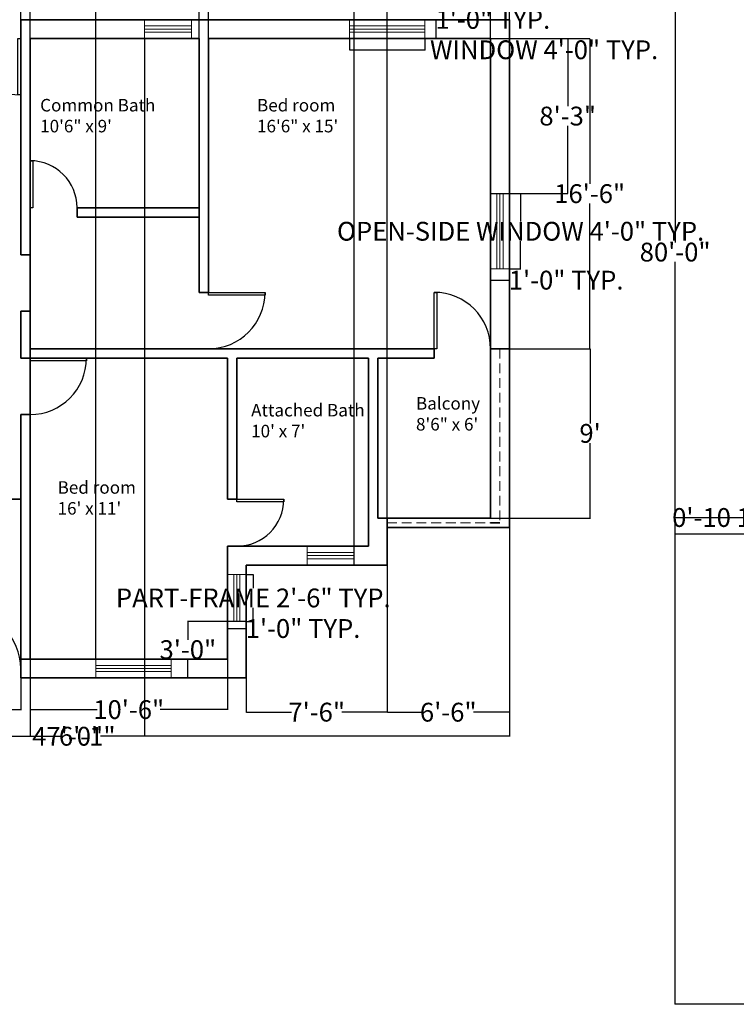
# Model space of a CAD drawing. Units: inches. Extents: x 2450 to 4494, y 1482 to 2597.
# Tile 2 of 7: x 2780 to 3238, y 1559 to 2188. Entities that reach past the tile are written whole.
import ezdxf

# ---------------------------------------------------------------- set-up
doc = ezdxf.new("R2010")
doc.units = ezdxf.units.IN
doc.header["$LTSCALE"] = 5
doc.header["$MEASUREMENT"] = 0
doc.linetypes.add('HIDDEN', pattern=[0.375, 0.25, -0.125])
for name, color, linetype, lineweight in [('A-ANNO-DIMS', 2, 'Continuous', 18), ('A-AREA-IDEN', 7, 'Continuous', 18), ('A-DOOR', 4, 'Continuous', 25), ('A-GLAZ', 4, 'Continuous', 18), ('A-WALL', 7, 'Continuous', 35), ('A-WALL-HIDN', 7, 'HIDDEN', 18)]:
    doc.layers.add(name, color=color, linetype=linetype, lineweight=lineweight)
doc.styles.get("Standard").update_dxf_attribs({"font": 'arial.ttf'})
doc.dimstyles.get("Standard").update_dxf_attribs({"dimtxt": 12, "dimasz": 0.18, "dimexe": 0.18, "dimexo": 0.0625, "dimgap": 0.09, "dimtad": 0, "dimtih": 1, "dimtoh": 1, "dimdec": 0, "dimzin": 0, "dimdsep": 46, "dimlunit": 3, "dimtxsty": 'Standard', "dimcen": 0.09, "dimadec": 0, "dimazin": 0, "dimtfac": 1, "dimtdec": 0, "dimtofl": 0, "dimtmove": 0, "dimatfit": 3, "dimfxl": 1, "dimtolj": 1, "dimtzin": 0, "dimarcsym": 0})

# ---------------------------------------------------------------- blocks, each defined once
blk = doc.blocks.new('*U2')
for p, q in [((0, 0), (0, -6)), ((36, 0), (36, -6))]:
    blk.add_line(p, q)
blk.add_lwpolyline([(0, 0), (0, 36), (1.75, 36), (1.75, 0)], close=True)
blk.add_arc((0, 0), 36, 0, 90)
blk = doc.blocks.new('*U3')
for p, q in [((0, 0), (0, -6)), ((30, 0), (30, -6))]:
    blk.add_line(p, q)
blk.add_lwpolyline([(0, 0), (0, 30), (1.75, 30), (1.75, 0)], close=True)
blk.add_arc((0, 0), 30, 0, 90)
blk = doc.blocks.new('*U5')
for p, q in [((-36, 0), (-36, 6)), ((0, 0), (0, 6))]:
    blk.add_line(p, q)
blk.add_lwpolyline([(0, 0), (0, -36), (-1.75, -36), (-1.75, 0)], close=True)
blk.add_arc((0, 0), 36, 180, 270)
blk = doc.blocks.new('*D6')
at = {"layer": 'A-ANNO-DIMS', "color": 0, "lineweight": -2, "ltscale": 5, "transparency": 16777216}
for p, q in [((2900.93, 2175.63), (2900.93, 2236.59)), ((2901.11, 2236.41), (2981.22, 2236.41)), ((3080.75, 2236.41), (3000.64, 2236.41)), ((3080.93, 2175.63), (3080.93, 2236.59))]:
    blk.add_line(p, q, dxfattribs=at)
at = {"layer": 'A-ANNO-DIMS', "color": 0, "ltscale": 5, "transparency": 16777216}
for points in [[(2901.11, 2236.44), (2901.11, 2236.38), (2900.93, 2236.41)], [(3080.75, 2236.44), (3080.75, 2236.38), (3080.93, 2236.41)]]:
    blk.add_solid(points, dxfattribs=at)
at = {"layer": 'Defpoints', "color": 0, "ltscale": 5, "transparency": 16777216}
for p in [(3080.93, 2236.41), (2900.93, 2175.57), (3080.93, 2175.57)]:
    blk.add_point(p, dxfattribs=at)
at = {"layer": 'A-ANNO-DIMS', "color": 0, "ltscale": 5, "transparency": 16777216, "insert": (2990.93, 2236.41), "char_height": 12, "attachment_point": 5}
blk.add_mtext("\\A1;15'", dxfattribs=at)
blk = doc.blocks.new('*D7')
at = {"layer": 'A-ANNO-DIMS', "color": 0, "lineweight": -2, "ltscale": 5, "transparency": 16777216}
for p, q in [((3080.93, 2175.63), (3080.93, 2236.59)), ((3081.11, 2236.41), (3081.88, 2236.41)), ((3092.75, 2236.41), (3091.98, 2236.41)), ((3092.93, 2175.63), (3092.93, 2236.59))]:
    blk.add_line(p, q, dxfattribs=at)
at = {"layer": 'A-ANNO-DIMS', "color": 0, "ltscale": 5, "transparency": 16777216}
for points in [[(3081.11, 2236.44), (3081.11, 2236.38), (3080.93, 2236.41)], [(3092.75, 2236.44), (3092.75, 2236.38), (3092.93, 2236.41)]]:
    blk.add_solid(points, dxfattribs=at)
at = {"layer": 'Defpoints', "color": 0, "ltscale": 5, "transparency": 16777216}
for p in [(3092.93, 2236.41), (3080.93, 2175.57), (3092.93, 2175.57)]:
    blk.add_point(p, dxfattribs=at)
at = {"layer": 'A-ANNO-DIMS', "color": 0, "ltscale": 5, "transparency": 16777216, "insert": (3086.93, 2236.41), "char_height": 12, "attachment_point": 5}
blk.add_mtext("\\A1;1'", dxfattribs=at)
blk = doc.blocks.new('*D8')
at = {"layer": 'A-ANNO-DIMS', "color": 0, "lineweight": -2, "ltscale": 5, "transparency": 16777216}
for p, q in [((2786.93, 2175.63), (2786.93, 2236.19)), ((2787.11, 2236.01), (2835.32, 2236.01)), ((2894.75, 2236.01), (2846.54, 2236.01)), ((2894.93, 2175.63), (2894.93, 2236.19))]:
    blk.add_line(p, q, dxfattribs=at)
at = {"layer": 'A-ANNO-DIMS', "color": 0, "ltscale": 5, "transparency": 16777216}
for points in [[(2787.11, 2236.04), (2787.11, 2235.98), (2786.93, 2236.01)], [(2894.75, 2236.04), (2894.75, 2235.98), (2894.93, 2236.01)]]:
    blk.add_solid(points, dxfattribs=at)
at = {"layer": 'Defpoints', "color": 0, "ltscale": 5, "transparency": 16777216}
for p in [(2894.93, 2236.01), (2786.93, 2175.57), (2894.93, 2175.57)]:
    blk.add_point(p, dxfattribs=at)
at = {"layer": 'A-ANNO-DIMS', "color": 0, "ltscale": 5, "transparency": 16777216, "insert": (2840.93, 2236.01), "char_height": 12, "attachment_point": 5}
blk.add_mtext("\\A1;9'", dxfattribs=at)
blk = doc.blocks.new('*D9')
at = {"layer": 'A-ANNO-DIMS', "color": 0, "lineweight": -2, "ltscale": 5, "transparency": 16777216}
for p, q in [((2894.93, 2175.63), (2894.93, 2251.28)), ((2895.11, 2251.1), (2900.75, 2251.1)), ((2900.93, 2175.63), (2900.93, 2251.28)), ((2900.93, 2251.1), (2901.11, 2251.1))]:
    blk.add_line(p, q, dxfattribs=at)
at = {"layer": 'A-ANNO-DIMS', "color": 0, "ltscale": 5, "transparency": 16777216}
for points in [[(2895.11, 2251.13), (2895.11, 2251.07), (2894.93, 2251.1)], [(2900.75, 2251.13), (2900.75, 2251.07), (2900.93, 2251.1)]]:
    blk.add_solid(points, dxfattribs=at)
at = {"layer": 'Defpoints', "color": 0, "ltscale": 5, "transparency": 16777216}
for p in [(2900.93, 2251.1), (2894.93, 2175.57), (2900.93, 2175.57)]:
    blk.add_point(p, dxfattribs=at)
at = {"layer": 'A-ANNO-DIMS', "color": 0, "ltscale": 5, "transparency": 16777216, "insert": (2908.13, 2251.1), "char_height": 12, "attachment_point": 5}
blk.add_mtext('\\A1;6"', dxfattribs=at)
blk = doc.blocks.new('*D10')
at = {"layer": 'A-ANNO-DIMS', "color": 0, "lineweight": -2, "ltscale": 5, "transparency": 16777216}
for p, q in [((2648.93, 2175.63), (2648.93, 2236.37)), ((2649.11, 2236.19), (2705.22, 2236.19)), ((2780.75, 2236.19), (2724.64, 2236.19)), ((2780.93, 2175.63), (2780.93, 2236.37))]:
    blk.add_line(p, q, dxfattribs=at)
at = {"layer": 'A-ANNO-DIMS', "color": 0, "ltscale": 5, "transparency": 16777216}
for points in [[(2649.11, 2236.22), (2649.11, 2236.16), (2648.93, 2236.19)], [(2780.75, 2236.22), (2780.75, 2236.16), (2780.93, 2236.19)]]:
    blk.add_solid(points, dxfattribs=at)
at = {"layer": 'Defpoints', "color": 0, "ltscale": 5, "transparency": 16777216}
for p in [(2780.93, 2236.19), (2648.93, 2175.57), (2780.93, 2175.57)]:
    blk.add_point(p, dxfattribs=at)
at = {"layer": 'A-ANNO-DIMS', "color": 0, "ltscale": 5, "transparency": 16777216, "insert": (2714.93, 2236.19), "char_height": 12, "attachment_point": 5}
blk.add_mtext("\\A1;11'", dxfattribs=at)
blk = doc.blocks.new('*D18')
at = {"layer": 'A-ANNO-DIMS', "color": 0, "lineweight": -2, "ltscale": 5, "transparency": 16777216}
for p, q in [((2648.93, 1779.51), (2648.93, 1747)), ((2780.93, 1779.51), (2780.93, 1747)), ((2649.11, 1747.18), (2705.22, 1747.18)), ((2780.75, 1747.18), (2724.64, 1747.18))]:
    blk.add_line(p, q, dxfattribs=at)
at = {"layer": 'A-ANNO-DIMS', "color": 0, "ltscale": 5, "transparency": 16777216}
for points in [[(2649.11, 1747.21), (2649.11, 1747.15), (2648.93, 1747.18)], [(2780.75, 1747.21), (2780.75, 1747.15), (2780.93, 1747.18)]]:
    blk.add_solid(points, dxfattribs=at)
at = {"layer": 'Defpoints', "color": 0, "ltscale": 5, "transparency": 16777216}
for p in [(2648.93, 1779.57), (2780.93, 1779.57), (2648.93, 1747.18)]:
    blk.add_point(p, dxfattribs=at)
at = {"layer": 'A-ANNO-DIMS', "color": 0, "ltscale": 5, "transparency": 16777216, "insert": (2714.93, 1747.18), "char_height": 12, "attachment_point": 5}
blk.add_mtext("\\A1;11'", dxfattribs=at)
blk = doc.blocks.new('*D19')
at = {"layer": 'A-ANNO-DIMS', "color": 0, "lineweight": -2, "ltscale": 5, "transparency": 16777216}
for p, q in [((2786.93, 1779.51), (2786.93, 1747.15)), ((2912.93, 1779.51), (2912.93, 1747.15)), ((2787.11, 1747.33), (2829.79, 1747.33)), ((2912.75, 1747.33), (2870.07, 1747.33))]:
    blk.add_line(p, q, dxfattribs=at)
at = {"layer": 'A-ANNO-DIMS', "color": 0, "ltscale": 5, "transparency": 16777216}
for points in [[(2787.11, 1747.36), (2787.11, 1747.3), (2786.93, 1747.33)], [(2912.75, 1747.36), (2912.75, 1747.3), (2912.93, 1747.33)]]:
    blk.add_solid(points, dxfattribs=at)
at = {"layer": 'Defpoints', "color": 0, "ltscale": 5, "transparency": 16777216}
for p in [(2786.93, 1779.57), (2912.93, 1779.57), (2912.93, 1747.33)]:
    blk.add_point(p, dxfattribs=at)
at = {"layer": 'A-ANNO-DIMS', "color": 0, "ltscale": 5, "transparency": 16777216, "insert": (2849.93, 1747.33), "char_height": 12, "attachment_point": 5}
blk.add_mtext('\\A1;10\'-6"', dxfattribs=at)
blk = doc.blocks.new('*D20')
at = {"layer": 'A-ANNO-DIMS', "color": 0, "lineweight": -2, "ltscale": 5, "transparency": 16777216}
for p, q in [((2924.93, 1839.51), (2924.93, 1745.52)), ((3014.93, 1839.51), (3014.93, 1745.52)), ((2925.11, 1745.7), (2953.94, 1745.7)), ((3014.75, 1745.7), (2985.92, 1745.7))]:
    blk.add_line(p, q, dxfattribs=at)
at = {"layer": 'A-ANNO-DIMS', "color": 0, "ltscale": 5, "transparency": 16777216}
for points in [[(2925.11, 1745.73), (2925.11, 1745.67), (2924.93, 1745.7)], [(3014.75, 1745.73), (3014.75, 1745.67), (3014.93, 1745.7)]]:
    blk.add_solid(points, dxfattribs=at)
at = {"layer": 'Defpoints', "color": 0, "ltscale": 5, "transparency": 16777216}
for p in [(2924.93, 1839.57), (3014.93, 1839.57), (3014.93, 1745.7)]:
    blk.add_point(p, dxfattribs=at)
at = {"layer": 'A-ANNO-DIMS', "color": 0, "ltscale": 5, "transparency": 16777216, "insert": (2969.93, 1745.7), "char_height": 12, "attachment_point": 5}
blk.add_mtext('\\A1;7\'-6"', dxfattribs=at)
blk = doc.blocks.new('*D21')
at = {"layer": 'A-ANNO-DIMS', "color": 0, "lineweight": -2, "ltscale": 5, "transparency": 16777216}
for p, q in [((3014.93, 1863.51), (3014.93, 1745.49)), ((3092.93, 1863.51), (3092.93, 1745.49)), ((3015.11, 1745.67), (3037.86, 1745.67)), ((3092.75, 1745.67), (3070, 1745.67))]:
    blk.add_line(p, q, dxfattribs=at)
at = {"layer": 'A-ANNO-DIMS', "color": 0, "ltscale": 5, "transparency": 16777216}
for points in [[(3015.11, 1745.7), (3015.11, 1745.64), (3014.93, 1745.67)], [(3092.75, 1745.7), (3092.75, 1745.64), (3092.93, 1745.67)]]:
    blk.add_solid(points, dxfattribs=at)
at = {"layer": 'Defpoints', "color": 0, "ltscale": 5, "transparency": 16777216}
for p in [(3014.93, 1863.57), (3092.93, 1863.57), (3014.93, 1745.67)]:
    blk.add_point(p, dxfattribs=at)
at = {"layer": 'A-ANNO-DIMS', "color": 0, "ltscale": 5, "transparency": 16777216, "insert": (3053.93, 1745.67), "char_height": 12, "attachment_point": 5}
blk.add_mtext('\\A1;6\'-6"', dxfattribs=at)
blk = doc.blocks.new('*D22')
at = {"layer": 'A-ANNO-DIMS', "color": 0, "lineweight": -2, "ltscale": 5, "transparency": 16777216}
for p, q in [((3080.99, 1977.57), (3144.66, 1977.57)), ((3144.48, 1977.39), (3144.48, 1929.79)), ((3144.48, 1869.75), (3144.48, 1917.35)), ((3080.99, 1869.57), (3144.66, 1869.57))]:
    blk.add_line(p, q, dxfattribs=at)
at = {"layer": 'A-ANNO-DIMS', "color": 0, "ltscale": 5, "transparency": 16777216}
for points in [[(3144.45, 1977.39), (3144.51, 1977.39), (3144.48, 1977.57)], [(3144.45, 1869.75), (3144.51, 1869.75), (3144.48, 1869.57)]]:
    blk.add_solid(points, dxfattribs=at)
at = {"layer": 'Defpoints', "color": 0, "ltscale": 5, "transparency": 16777216}
for p in [(3080.93, 1977.57), (3144.48, 1977.57), (3080.93, 1869.57)]:
    blk.add_point(p, dxfattribs=at)
at = {"layer": 'A-ANNO-DIMS', "color": 0, "ltscale": 5, "transparency": 16777216, "insert": (3144.48, 1923.57), "char_height": 12, "attachment_point": 5}
blk.add_mtext("\\A1;9'", dxfattribs=at)
blk = doc.blocks.new('*D23')
at = {"layer": 'A-ANNO-DIMS', "color": 0, "lineweight": -2, "ltscale": 5, "transparency": 16777216}
for p, q in [((3080.99, 2175.57), (3144.41, 2175.57)), ((3144.23, 2175.39), (3144.23, 2082.79)), ((3144.23, 1977.75), (3144.23, 2070.35)), ((3080.99, 1977.57), (3144.41, 1977.57))]:
    blk.add_line(p, q, dxfattribs=at)
at = {"layer": 'A-ANNO-DIMS', "color": 0, "ltscale": 5, "transparency": 16777216}
for points in [[(3144.2, 2175.39), (3144.26, 2175.39), (3144.23, 2175.57)], [(3144.2, 1977.75), (3144.26, 1977.75), (3144.23, 1977.57)]]:
    blk.add_solid(points, dxfattribs=at)
at = {"layer": 'Defpoints', "color": 0, "ltscale": 5, "transparency": 16777216}
for p in [(3080.93, 2175.57), (3080.93, 1977.57), (3144.23, 1977.57)]:
    blk.add_point(p, dxfattribs=at)
at = {"layer": 'A-ANNO-DIMS', "color": 0, "ltscale": 5, "transparency": 16777216, "insert": (3144.23, 2076.57), "char_height": 12, "attachment_point": 5}
blk.add_mtext('\\A1;16\'-6"', dxfattribs=at)
blk = doc.blocks.new('WIN-30-FRAME')
for p, q in [((0, 0), (0, 12)), ((0, 12), (30, 12)), ((30, 8), (0, 8)), ((30, 12), (30, 0)), ((30, 6), (0, 6)), ((30, 4), (0, 4)), ((30, 0), (0, 0))]:
    blk.add_line(p, q)
blk = doc.blocks.new('WIN-48-FRAME')
for p, q in [((48, 12), (0, 12)), ((0, 12), (0, 0)), ((48, 8), (0, 8)), ((48, 0), (48, 12)), ((48, 6), (0, 6)), ((48, 4), (0, 4)), ((0, 0), (48, 0))]:
    blk.add_line(p, q)
blk = doc.blocks.new('WIN-30-PART-FRAME')
for p, q in [((12, 30), (0, 30)), ((0, 30), (0, 0)), ((4, 30), (4, 0)), ((6, 30), (6, 0)), ((8, 30), (8, 0)), ((12, 6), (12, 30)), ((0, 0), (12, 0))]:
    blk.add_line(p, q)
blk = doc.blocks.new('WIN-48-PART-FRAME')
for p, q in [((48, 12), (0, 12)), ((0, 12), (0, 0)), ((48, 8), (0, 8)), ((48, 0), (48, 12)), ((48, 6), (0, 6)), ((48, 4), (0, 4)), ((24, 0), (48, 0))]:
    blk.add_line(p, q)
blk = doc.blocks.new('WIN-48-OPEN-SIDE')
for p, q in [((0, 48), (12, 48)), ((4, 48), (4, 0)), ((6, 48), (6, 0)), ((8, 48), (8, 0)), ((12, 48), (12, 0)), ((12, 0), (0, 0))]:
    blk.add_line(p, q)
blk = doc.blocks.new('*D41')
at = {"layer": 'A-ANNO-DIMS', "color": 0, "lineweight": -2, "ltscale": 5, "transparency": 16777216}
for p, q in [((2990.93, 2175.51), (2990.93, 2168.19)), ((3038.93, 2175.51), (3038.93, 2168.19)), ((2991.11, 2168.37), (3038.75, 2168.37)), ((3038.93, 2168.37), (3039.11, 2168.37))]:
    blk.add_line(p, q, dxfattribs=at)
at = {"layer": 'A-ANNO-DIMS', "color": 0, "ltscale": 5, "transparency": 16777216}
for points in [[(2991.11, 2168.4), (2991.11, 2168.34), (2990.93, 2168.37)], [(3038.75, 2168.4), (3038.75, 2168.34), (3038.93, 2168.37)]]:
    blk.add_solid(points, dxfattribs=at)
at = {"layer": 'Defpoints', "color": 0, "ltscale": 5, "transparency": 16777216}
for p in [(2990.93, 2175.57), (3038.93, 2175.57), (3038.93, 2168.37)]:
    blk.add_point(p, dxfattribs=at)
at = {"layer": 'A-ANNO-DIMS', "color": 0, "ltscale": 5, "transparency": 16777216, "insert": (3115.13, 2168.37), "char_height": 12, "attachment_point": 5}
blk.add_mtext('\\A1;WINDOW 4\'-0" TYP.', dxfattribs=at)
blk = doc.blocks.new('*D42')
at = {"layer": 'A-ANNO-DIMS', "color": 0, "lineweight": -2, "ltscale": 5, "transparency": 16777216}
for p, q in [((3038.99, 2187.57), (3046.31, 2187.57)), ((3046.13, 2187.57), (3046.13, 2187.75)), ((3046.13, 2187.75), (3046.31, 2187.75)), ((3046.13, 2175.75), (3046.13, 2187.39)), ((3038.99, 2175.57), (3046.31, 2175.57))]:
    blk.add_line(p, q, dxfattribs=at)
at = {"layer": 'A-ANNO-DIMS', "color": 0, "ltscale": 5, "transparency": 16777216}
for points in [[(3046.1, 2187.39), (3046.16, 2187.39), (3046.13, 2187.57)], [(3046.1, 2175.75), (3046.16, 2175.75), (3046.13, 2175.57)]]:
    blk.add_solid(points, dxfattribs=at)
at = {"layer": 'Defpoints', "color": 0, "ltscale": 5, "transparency": 16777216}
for p in [(3038.93, 2187.57), (3046.13, 2187.57), (3038.93, 2175.57)]:
    blk.add_point(p, dxfattribs=at)
at = {"layer": 'A-ANNO-DIMS', "color": 0, "ltscale": 5, "transparency": 16777216, "insert": (3082.41, 2187.75), "char_height": 12, "attachment_point": 5}
blk.add_mtext('\\A1;1\'-0" TYP.', dxfattribs=at)
blk = doc.blocks.new('*D43')
at = {"layer": 'A-ANNO-DIMS', "color": 0, "lineweight": -2, "ltscale": 5, "transparency": 16777216}
for p, q in [((2924.99, 1833.57), (2929.61, 1833.57)), ((2929.43, 1833.39), (2929.43, 1824.79)), ((2929.43, 1803.75), (2929.43, 1812.35)), ((2924.99, 1803.57), (2929.61, 1803.57))]:
    blk.add_line(p, q, dxfattribs=at)
at = {"layer": 'A-ANNO-DIMS', "color": 0, "ltscale": 5, "transparency": 16777216}
for points in [[(2929.4, 1833.39), (2929.46, 1833.39), (2929.43, 1833.57)], [(2929.4, 1803.75), (2929.46, 1803.75), (2929.43, 1803.57)]]:
    blk.add_solid(points, dxfattribs=at)
at = {"layer": 'Defpoints', "color": 0, "ltscale": 5, "transparency": 16777216}
for p in [(2924.93, 1833.57), (2929.43, 1833.57), (2924.93, 1803.57)]:
    blk.add_point(p, dxfattribs=at)
at = {"layer": 'A-ANNO-DIMS', "color": 0, "ltscale": 5, "transparency": 16777216, "insert": (2929.43, 1818.57), "char_height": 12, "attachment_point": 5}
blk.add_mtext('\\A1;PART-FRAME 2\'-6" TYP.', dxfattribs=at)
blk = doc.blocks.new('*D44')
at = {"layer": 'A-ANNO-DIMS', "color": 0, "lineweight": -2, "ltscale": 5, "transparency": 16777216}
for p, q in [((2912.93, 1803.51), (2912.93, 1798.89)), ((2924.93, 1803.51), (2924.93, 1798.89)), ((2913.11, 1799.07), (2924.75, 1799.07)), ((2924.93, 1799.07), (2925.11, 1799.07))]:
    blk.add_line(p, q, dxfattribs=at)
at = {"layer": 'A-ANNO-DIMS', "color": 0, "ltscale": 5, "transparency": 16777216}
for points in [[(2913.11, 1799.1), (2913.11, 1799.04), (2912.93, 1799.07)], [(2924.75, 1799.1), (2924.75, 1799.04), (2924.93, 1799.07)]]:
    blk.add_solid(points, dxfattribs=at)
at = {"layer": 'Defpoints', "color": 0, "ltscale": 5, "transparency": 16777216}
for p in [(2912.93, 1803.57), (2924.93, 1803.57), (2924.93, 1799.07)]:
    blk.add_point(p, dxfattribs=at)
at = {"layer": 'A-ANNO-DIMS', "color": 0, "ltscale": 5, "transparency": 16777216, "insert": (2961.21, 1799.07), "char_height": 12, "attachment_point": 5}
blk.add_mtext('\\A1;1\'-0" TYP.', dxfattribs=at)
blk = doc.blocks.new('*D47')
at = {"layer": 'A-ANNO-DIMS', "color": 0, "lineweight": -2, "ltscale": 5, "transparency": 16777216}
for p, q in [((3092.99, 2076.57), (3100.31, 2076.57)), ((3100.13, 2076.39), (3100.13, 2058.87)), ((3100.13, 2028.75), (3100.13, 2046.27)), ((3092.99, 2028.57), (3100.31, 2028.57))]:
    blk.add_line(p, q, dxfattribs=at)
at = {"layer": 'A-ANNO-DIMS', "color": 0, "ltscale": 5, "transparency": 16777216}
for points in [[(3100.1, 2076.39), (3100.16, 2076.39), (3100.13, 2076.57)], [(3100.1, 2028.75), (3100.16, 2028.75), (3100.13, 2028.57)]]:
    blk.add_solid(points, dxfattribs=at)
at = {"layer": 'Defpoints', "color": 0, "ltscale": 5, "transparency": 16777216}
for p in [(3092.93, 2076.57), (3100.13, 2076.57), (3092.93, 2028.57)]:
    blk.add_point(p, dxfattribs=at)
at = {"layer": 'A-ANNO-DIMS', "color": 0, "ltscale": 5, "transparency": 16777216, "insert": (3100.13, 2052.57), "char_height": 12, "attachment_point": 5}
blk.add_mtext('\\A1;OPEN-SIDE WINDOW 4\'-0" TYP.', dxfattribs=at)
blk = doc.blocks.new('*D48')
at = {"layer": 'A-ANNO-DIMS', "color": 0, "lineweight": -2, "ltscale": 5, "transparency": 16777216}
for p, q in [((3080.93, 2028.51), (3080.93, 2021.19)), ((3092.93, 2028.51), (3092.93, 2021.19)), ((3081.11, 2021.37), (3092.75, 2021.37)), ((3092.93, 2021.37), (3093.11, 2021.37))]:
    blk.add_line(p, q, dxfattribs=at)
at = {"layer": 'A-ANNO-DIMS', "color": 0, "ltscale": 5, "transparency": 16777216}
for points in [[(3081.11, 2021.4), (3081.11, 2021.34), (3080.93, 2021.37)], [(3092.75, 2021.4), (3092.75, 2021.34), (3092.93, 2021.37)]]:
    blk.add_solid(points, dxfattribs=at)
at = {"layer": 'Defpoints', "color": 0, "ltscale": 5, "transparency": 16777216}
for p in [(3080.93, 2028.57), (3092.93, 2028.57), (3092.93, 2021.37)]:
    blk.add_point(p, dxfattribs=at)
at = {"layer": 'A-ANNO-DIMS', "color": 0, "ltscale": 5, "transparency": 16777216, "insert": (3129.21, 2021.37), "char_height": 12, "attachment_point": 5}
blk.add_mtext('\\A1;1\'-0" TYP.', dxfattribs=at)
blk = doc.blocks.new('*D69')
at = {"layer": 'A-ANNO-DIMS', "color": 0, "lineweight": -2, "ltscale": 5, "transparency": 16777216}
for p, q in [((2528.93, 1869.51), (2528.93, 1730.14)), ((3092.93, 1863.51), (3092.93, 1730.14)), ((2529.11, 1730.32), (2789.99, 1730.32)), ((3092.75, 1730.32), (2831.87, 1730.32))]:
    blk.add_line(p, q, dxfattribs=at)
at = {"layer": 'A-ANNO-DIMS', "color": 0, "ltscale": 5, "transparency": 16777216}
for points in [[(2529.11, 1730.35), (2529.11, 1730.29), (2528.93, 1730.32)], [(3092.75, 1730.35), (3092.75, 1730.29), (3092.93, 1730.32)]]:
    blk.add_solid(points, dxfattribs=at)
at = {"layer": 'Defpoints', "color": 0, "ltscale": 5, "transparency": 16777216}
for p in [(2528.93, 1869.57), (3092.93, 1863.57), (3092.93, 1730.32)]:
    blk.add_point(p, dxfattribs=at)
at = {"layer": 'A-ANNO-DIMS', "color": 0, "ltscale": 5, "transparency": 16777216, "insert": (2810.93, 1730.32), "char_height": 12, "attachment_point": 5}
blk.add_mtext('\\A1;47\'-0"', dxfattribs=at)
blk = doc.blocks.new('*D72')
at = {"layer": 'A-ANNO-DIMS', "color": 0, "lineweight": -2, "ltscale": 5, "transparency": 16777216}
for p, q in [((3426.23, 2519.27), (3198.61, 2519.27)), ((3198.79, 2519.09), (3198.79, 2045.48)), ((3198.79, 1559.45), (3198.79, 2033.05)), ((3426.23, 1559.27), (3198.61, 1559.27))]:
    blk.add_line(p, q, dxfattribs=at)
at = {"layer": 'A-ANNO-DIMS', "color": 0, "ltscale": 5, "transparency": 16777216}
for points in [[(3198.76, 2519.09), (3198.82, 2519.09), (3198.79, 2519.27)], [(3198.76, 1559.45), (3198.82, 1559.45), (3198.79, 1559.27)]]:
    blk.add_solid(points, dxfattribs=at)
at = {"layer": 'Defpoints', "color": 0, "ltscale": 5, "transparency": 16777216}
for p in [(3198.79, 2519.27), (3426.29, 2519.27), (3426.29, 1559.27)]:
    blk.add_point(p, dxfattribs=at)
at = {"layer": 'A-ANNO-DIMS', "color": 0, "ltscale": 5, "transparency": 16777216, "insert": (3198.79, 2039.27), "char_height": 12, "attachment_point": 5}
blk.add_mtext('\\A1;80\'-0"', dxfattribs=at)
blk = doc.blocks.new('*D76')
at = {"layer": 'A-ANNO-DIMS', "color": 0, "lineweight": -2, "ltscale": 5, "transparency": 16777216}
for p, q in [((2786.93, 2175.51), (2786.93, 1730.14)), ((2859.92, 2175.51), (2859.92, 1730.14)), ((2787.11, 1730.32), (2807.35, 1730.32)), ((2859.74, 1730.32), (2839.5, 1730.32))]:
    blk.add_line(p, q, dxfattribs=at)
at = {"layer": 'A-ANNO-DIMS', "color": 0, "ltscale": 5, "transparency": 16777216}
for points in [[(2787.11, 1730.35), (2787.11, 1730.29), (2786.93, 1730.32)], [(2859.74, 1730.35), (2859.74, 1730.29), (2859.92, 1730.32)]]:
    blk.add_solid(points, dxfattribs=at)
at = {"layer": 'Defpoints', "color": 0, "ltscale": 5, "transparency": 16777216}
for p in [(2786.93, 2175.57), (2859.92, 2175.57), (2859.92, 1730.32)]:
    blk.add_point(p, dxfattribs=at)
at = {"layer": 'A-ANNO-DIMS', "color": 0, "ltscale": 5, "transparency": 16777216, "insert": (2823.43, 1730.32), "char_height": 12, "attachment_point": 5}
blk.add_mtext('\\A1;6\'-1"', dxfattribs=at)
blk = doc.blocks.new('*D78')
at = {"layer": 'A-ANNO-DIMS', "color": 0, "lineweight": -2, "ltscale": 5, "transparency": 16777216}
for p, q in [((3080.99, 2175.57), (3130.36, 2175.57)), ((3130.18, 2175.39), (3130.18, 2132.29)), ((3130.18, 2076.75), (3130.18, 2119.85)), ((3080.99, 2076.57), (3130.36, 2076.57))]:
    blk.add_line(p, q, dxfattribs=at)
at = {"layer": 'A-ANNO-DIMS', "color": 0, "ltscale": 5, "transparency": 16777216}
for points in [[(3130.15, 2175.39), (3130.21, 2175.39), (3130.18, 2175.57)], [(3130.15, 2076.75), (3130.21, 2076.75), (3130.18, 2076.57)]]:
    blk.add_solid(points, dxfattribs=at)
at = {"layer": 'Defpoints', "color": 0, "ltscale": 5, "transparency": 16777216}
for p in [(3080.93, 2175.57), (3080.93, 2076.57), (3130.18, 2076.57)]:
    blk.add_point(p, dxfattribs=at)
at = {"layer": 'A-ANNO-DIMS', "color": 0, "ltscale": 5, "transparency": 16777216, "insert": (3130.18, 2126.07), "char_height": 12, "attachment_point": 5}
blk.add_mtext('\\A1;8\'-3"', dxfattribs=at)
blk = doc.blocks.new('*D79')
at = {"layer": 'A-ANNO-DIMS', "color": 0, "lineweight": -2, "ltscale": 5, "transparency": 16777216}
for p, q in [((2786.93, 1779.63), (2786.93, 2225)), ((2787.11, 2224.82), (2791.9, 2224.82)), ((2828.75, 2224.82), (2823.97, 2224.82)), ((2828.93, 1779.63), (2828.93, 2225))]:
    blk.add_line(p, q, dxfattribs=at)
at = {"layer": 'A-ANNO-DIMS', "color": 0, "ltscale": 5, "transparency": 16777216}
for points in [[(2787.11, 2224.85), (2787.11, 2224.79), (2786.93, 2224.82)], [(2828.75, 2224.85), (2828.75, 2224.79), (2828.93, 2224.82)]]:
    blk.add_solid(points, dxfattribs=at)
at = {"layer": 'Defpoints', "color": 0, "ltscale": 5, "transparency": 16777216}
for p in [(2828.93, 2224.82), (2786.93, 1779.57), (2828.93, 1779.57)]:
    blk.add_point(p, dxfattribs=at)
at = {"layer": 'A-ANNO-DIMS', "color": 0, "ltscale": 5, "transparency": 16777216, "insert": (2807.93, 2224.82), "char_height": 12, "attachment_point": 5}
blk.add_mtext('\\A1;3\'-6"', dxfattribs=at)
blk = doc.blocks.new('*D80')
at = {"layer": 'A-ANNO-DIMS', "color": 0, "lineweight": -2, "ltscale": 5, "transparency": 16777216}
for p, q in [((2924.87, 1803.57), (2887.5, 1803.57)), ((2887.68, 1803.39), (2887.68, 1791.79)), ((2887.68, 1767.75), (2887.68, 1779.35)), ((2924.87, 1767.57), (2887.5, 1767.57))]:
    blk.add_line(p, q, dxfattribs=at)
at = {"layer": 'A-ANNO-DIMS', "color": 0, "ltscale": 5, "transparency": 16777216}
for points in [[(2887.65, 1803.39), (2887.71, 1803.39), (2887.68, 1803.57)], [(2887.65, 1767.75), (2887.71, 1767.75), (2887.68, 1767.57)]]:
    blk.add_solid(points, dxfattribs=at)
at = {"layer": 'Defpoints', "color": 0, "ltscale": 5, "transparency": 16777216}
for p in [(2887.68, 1803.57), (2924.93, 1803.57), (2924.93, 1767.57)]:
    blk.add_point(p, dxfattribs=at)
at = {"layer": 'A-ANNO-DIMS', "color": 0, "ltscale": 5, "transparency": 16777216, "insert": (2887.68, 1785.57), "char_height": 12, "attachment_point": 5}
blk.add_mtext('\\A1;3\'-0"', dxfattribs=at)
blk = doc.blocks.new('*D81')
at = {"layer": 'A-ANNO-DIMS', "color": 0, "lineweight": -2, "ltscale": 5, "transparency": 16777216}
for p, q in [((2993.93, 1839.63), (2993.93, 2225)), ((2994.11, 2224.82), (3014.75, 2224.82)), ((3014.93, 1839.63), (3014.93, 2225)), ((3014.93, 2224.82), (3015.11, 2224.82))]:
    blk.add_line(p, q, dxfattribs=at)
at = {"layer": 'A-ANNO-DIMS', "color": 0, "ltscale": 5, "transparency": 16777216}
for points in [[(2994.11, 2224.85), (2994.11, 2224.79), (2993.93, 2224.82)], [(3014.75, 2224.85), (3014.75, 2224.79), (3014.93, 2224.82)]]:
    blk.add_solid(points, dxfattribs=at)
at = {"layer": 'Defpoints', "color": 0, "ltscale": 5, "transparency": 16777216}
for p in [(3014.93, 2224.82), (2993.93, 1839.57), (3014.93, 1839.57)]:
    blk.add_point(p, dxfattribs=at)
at = {"layer": 'A-ANNO-DIMS', "color": 0, "ltscale": 5, "transparency": 16777216, "insert": (3030.59, 2224.82), "char_height": 12, "attachment_point": 5}
blk.add_mtext('\\A1;1\'-9"', dxfattribs=at)
blk = doc.blocks.new('*D86')
at = {"layer": 'A-ANNO-DIMS', "color": 0, "lineweight": -2, "ltscale": 5, "transparency": 16777216}
for p, q in [((3466.68, 1869.72), (3198.61, 1869.72)), ((3198.79, 1869.72), (3198.79, 1869.9)), ((3198.79, 1869.9), (3198.97, 1869.9)), ((3198.79, 1859.45), (3198.79, 1869.54)), ((3456.23, 1859.27), (3198.61, 1859.27))]:
    blk.add_line(p, q, dxfattribs=at)
at = {"layer": 'A-ANNO-DIMS', "color": 0, "ltscale": 5, "transparency": 16777216}
for points in [[(3198.76, 1869.54), (3198.82, 1869.54), (3198.79, 1869.72)], [(3198.76, 1859.45), (3198.82, 1859.45), (3198.79, 1859.27)]]:
    blk.add_solid(points, dxfattribs=at)
at = {"layer": 'Defpoints', "color": 0, "ltscale": 5, "transparency": 16777216}
for p in [(3198.79, 1869.72), (3466.74, 1869.72), (3456.29, 1859.27)]:
    blk.add_point(p, dxfattribs=at)
at = {"layer": 'A-ANNO-DIMS', "color": 0, "ltscale": 5, "transparency": 16777216, "insert": (3233.65, 1869.9), "char_height": 12, "attachment_point": 5}
blk.add_mtext('\\A1;0\'-10 1/2"', dxfattribs=at)

msp = doc.modelspace()

# ---------------------------------------------------------------- linework, layer by layer
at = {"layer": 'A-WALL'}
for p, q in [((3092.93, 2187.57), (2780.93, 2187.57)), ((2780.93, 2175.57), (2780.93, 2187.57)), ((3092.93, 1863.57), (3092.93, 2187.57)), ((2780.93, 2175.57), (2780.93, 2037.57)), ((2786.93, 2175.57), (2786.93, 2067.57)), ((2894.93, 2175.57), (2786.93, 2175.57)), ((2894.93, 2175.57), (2894.93, 2013.57)), ((3080.93, 2175.57), (2900.93, 2175.57)), ((2900.93, 2175.57), (2900.93, 2013.57)), ((3080.93, 1977.57), (3080.93, 2175.57)), ((2786.93, 2067.57), (2786.93, 2061.57)), ((2894.93, 2067.57), (2816.93, 2067.57)), ((2816.93, 2067.57), (2816.93, 2061.57)), ((2786.93, 2061.57), (2786.93, 2037.57)), ((2894.93, 2061.57), (2816.93, 2061.57)), ((2786.93, 2037.57), (2780.93, 2037.57)), ((2894.93, 2013.57), (2900.93, 2013.57)), ((2786.93, 2001.57), (2780.93, 2001.57)), ((2780.93, 2001.57), (2780.93, 1971.57)), ((2786.93, 2001.57), (2786.93, 1977.57)), ((2894.93, 1977.57), (2786.93, 1977.57)), ((2894.93, 1977.57), (2900.93, 1977.57)), ((3044.93, 1977.57), (2900.93, 1977.57)), ((3044.93, 1977.57), (3044.93, 1971.57)), ((3080.93, 1977.57), (3080.93, 1971.57)), ((3080.93, 1977.57), (3092.93, 1977.57)), ((2786.93, 1971.57), (2780.93, 1971.57)), ((2894.93, 1971.57), (2786.93, 1971.57)), ((2900.93, 1971.57), (2894.93, 1971.57)), ((2912.93, 1971.57), (2900.93, 1971.57)), ((2912.93, 1881.57), (2912.93, 1971.57)), ((3002.93, 1971.57), (2918.93, 1971.57)), ((2918.93, 1881.57), (2918.93, 1971.57)), ((3002.93, 1851.57), (3002.93, 1971.57)), ((3044.93, 1971.57), (3008.93, 1971.57)), ((3008.93, 1869.57), (3008.93, 1971.57)), ((3080.93, 1869.57), (3080.93, 1971.57)), ((2786.93, 1935.57), (2780.93, 1935.57)), ((2780.93, 1935.57), (2780.93, 1779.57)), ((2786.93, 1935.57), (2786.93, 1779.57)), ((2780.93, 1881.57), (2648.93, 1881.57)), ((2918.93, 1881.57), (2912.93, 1881.57)), ((3080.93, 1869.57), (3008.93, 1869.57)), ((3014.93, 1863.57), (3014.93, 1869.57)), ((3080.93, 1866.57), (3086.93, 1866.57)), ((3080.93, 1863.57), (3014.93, 1863.57)), ((3014.93, 1839.57), (3014.93, 1863.57)), ((3080.93, 1863.57), (3092.93, 1863.57)), ((2912.93, 1779.57), (2912.93, 1851.57)), ((2918.93, 1851.57), (2912.93, 1851.57)), ((3002.93, 1851.57), (2918.93, 1851.57)), ((3002.93, 1839.57), (2924.93, 1839.57)), ((2924.93, 1779.57), (2924.93, 1839.57)), ((3002.93, 1839.57), (3014.93, 1839.57)), ((2780.93, 1779.57), (2912.93, 1779.57)), ((2780.93, 1779.57), (2780.93, 1767.57)), ((2924.93, 1779.57), (2924.93, 1767.57)), ((2780.93, 1767.57), (2924.93, 1767.57))]:
    msp.add_line(p, q, dxfattribs=at)
at = {"layer": 'A-WALL-HIDN', "ltscale": 5}
for p, q in [((3086.93, 1977.57), (3086.93, 1866.57)), ((3014.93, 1866.57), (3080.93, 1866.57))]:
    msp.add_line(p, q, dxfattribs=at)

# ---------------------------------------------------------------- block references
at = {"layer": 'A-DOOR'}
for name, p in [('*U5', (2780.93, 2175.57)), ('*U3', (2786.93, 2067.57)), ('*U2', (3044.93, 1977.57)), ('*U2', (2744.93, 1773.57))]:
    msp.add_blockref(name, p, dxfattribs=at)
at = {"layer": 'A-DOOR', "rotation": 270}
for name, p in [('*U2', (2900.93, 2013.57)), ('*U2', (2786.93, 1971.57)), ('*U3', (2918.93, 1881.57))]:
    msp.add_blockref(name, p, dxfattribs=at)
at = {"layer": 'A-GLAZ'}
for name, p in [('WIN-30-FRAME', (2859.92, 2175.57)), ('WIN-48-FRAME', (2990.93, 2175.57)), ('WIN-48-OPEN-SIDE', (3080.93, 2028.57)), ('WIN-30-PART-FRAME', (2912.93, 1803.57)), ('WIN-48-PART-FRAME', (2828.93, 1767.57))]:
    msp.add_blockref(name, p, dxfattribs=at)
at = {"layer": 'A-GLAZ', "rotation": 180}
msp.add_blockref('WIN-30-FRAME', (2993.93, 1851.57), dxfattribs=at)

# ---------------------------------------------------------------- texts
at = {"layer": 'A-AREA-IDEN', "char_height": 8, "attachment_point": 1}
for s, insert in [('Common Bath\\P10\'6" x 9\'', (2793.36, 2137.01)), ('Bed room\\P16\'6" x 15\'', (2931.83, 2137.01)), ("Attached Bath\\P10' x 7'", (2928.07, 1942.4)), ('Balcony\\P8\'6" x 6\'', (3033.33, 1946.75)), ("Bed room\\P16' x 11'", (2804.5, 1893.08))]:
    msp.add_mtext_dynamic_manual_height_columns(s, width=155.5618, gutter_width=1, heights=[0], dxfattribs=dict(at, insert=insert))

# ---------------------------------------------------------------- dimensions: what is measured, and where the dimension line sits
at = {"layer": 'A-ANNO-DIMS', "ltscale": 5}
for base, p1, p2, override, picture, middle in [((3198.79, 2519.27), (3426.29, 1559.27), (3426.29, 2519.27), {"dimdec": 1, "dimlfac": 1, "dimrnd": 0, "dimzin": 1, "dimdsep": 46, "dimlunit": 4, "dimfrac": 2}, '*D72', (3198.79, 2039.27)), ((3144.23, 1977.57), (3080.93, 2175.57), (3080.93, 1977.57), {"dimclrd": 0, "dimclre": 0, "dimclrt": 0}, '*D23', (3144.23, 2076.57)), ((3130.18, 2076.57), (3080.93, 2175.57), (3080.93, 2076.57), {"dimdec": 1, "dimlfac": 1, "dimrnd": 0, "dimzin": 1, "dimdsep": 46, "dimlunit": 4, "dimfrac": 2}, '*D78', (3130.18, 2126.07)), ((3144.48, 1977.57), (3080.93, 1869.57), (3080.93, 1977.57), {"dimclrd": 0, "dimclre": 0, "dimclrt": 0}, '*D22', (3144.48, 1923.57)), ((3198.7899, 1869.7226), (3456.2899, 1859.2657), (3466.7402, 1869.7226), {"dimdec": 1, "dimlfac": 1, "dimrnd": 0, "dimzin": 1, "dimdsep": 46, "dimlunit": 4, "dimfrac": 2}, '*D86', (3233.652, 1869.9026)), ((2887.68, 1803.57), (2924.93, 1767.57), (2924.93, 1803.57), {"dimdec": 1, "dimlfac": 1, "dimrnd": 0, "dimzin": 1, "dimdsep": 46, "dimlunit": 4, "dimfrac": 2}, '*D80', (2887.68, 1785.57))]:
    dim = msp.add_linear_dim(base=base, p1=p1, p2=p2, angle=90, dimstyle='Standard', override=override, dxfattribs=at)
    dim.commit()
    dim.dimension.update_dxf_attribs({"geometry": picture, "text_midpoint": middle})
for base, p1, p2, override, picture, middle in [((2900.93, 2251.1), (2894.93, 2175.57), (2900.93, 2175.57), {"dimclrd": 0, "dimclre": 0, "dimclrt": 0}, '*D9', (2908.13, 2251.1)), ((2780.93, 2236.19), (2648.93, 2175.57), (2780.93, 2175.57), {"dimclrd": 0, "dimclre": 0, "dimclrt": 0}, '*D10', (2714.93, 2236.19)), ((2894.93, 2236.01), (2786.93, 2175.57), (2894.93, 2175.57), {"dimclrd": 0, "dimclre": 0, "dimclrt": 0}, '*D8', (2840.93, 2236.01)), ((3080.93, 2236.41), (2900.93, 2175.57), (3080.93, 2175.57), {"dimclrd": 0, "dimclre": 0, "dimclrt": 0}, '*D6', (2990.93, 2236.41)), ((3092.93, 2236.41), (3080.93, 2175.57), (3092.93, 2175.57), {"dimclrd": 0, "dimclre": 0, "dimclrt": 0}, '*D7', (3086.93, 2236.41)), ((2828.93, 2224.82), (2786.93, 1779.57), (2828.93, 1779.57), {"dimdec": 1, "dimlfac": 1, "dimrnd": 0, "dimzin": 1, "dimdsep": 46, "dimlunit": 4, "dimfrac": 2}, '*D79', (2807.93, 2224.82)), ((3014.93, 2224.82), (2993.93, 1839.57), (3014.93, 1839.57), {"dimdec": 1, "dimlfac": 1, "dimrnd": 0, "dimzin": 1, "dimdsep": 46, "dimlunit": 4, "dimfrac": 2}, '*D81', (3030.59, 2224.82)), ((2859.92, 1730.32), (2786.93, 2175.57), (2859.92, 2175.57), {"dimdec": 1, "dimlfac": 1, "dimrnd": 0, "dimzin": 1, "dimdsep": 46, "dimlunit": 4, "dimfrac": 2}, '*D76', (2823.43, 1730.32)), ((3092.93, 1730.32), (2528.93, 1869.57), (3092.93, 1863.57), {"dimdec": 1, "dimlfac": 1, "dimrnd": 0, "dimzin": 1, "dimdsep": 46, "dimlunit": 4, "dimfrac": 2}, '*D69', (2810.93, 1730.32)), ((3014.93, 1745.67), (3092.93, 1863.57), (3014.93, 1863.57), {"dimclrd": 0, "dimclre": 0, "dimclrt": 0}, '*D21', (3053.93, 1745.67)), ((3014.93, 1745.7), (2924.93, 1839.57), (3014.93, 1839.57), {"dimclrd": 0, "dimclre": 0, "dimclrt": 0}, '*D20', (2969.93, 1745.7)), ((2648.93, 1747.18), (2780.93, 1779.57), (2648.93, 1779.57), {"dimclrd": 0, "dimclre": 0, "dimclrt": 0}, '*D18', (2714.93, 1747.18)), ((2912.93, 1747.33), (2786.93, 1779.57), (2912.93, 1779.57), {"dimclrd": 0, "dimclre": 0, "dimclrt": 0}, '*D19', (2849.93, 1747.33))]:
    dim = msp.add_linear_dim(base=base, p1=p1, p2=p2, dimstyle='Standard', override=override, dxfattribs=at)
    dim.commit()
    dim.dimension.update_dxf_attribs({"geometry": picture, "text_midpoint": middle})
for base, p1, p2, text, picture, middle in [((3046.13, 2187.57), (3038.93, 2175.57), (3038.93, 2187.57), '<> TYP.', '*D42', (3082.41, 2187.75)), ((3100.13, 2076.57), (3092.93, 2028.57), (3092.93, 2076.57), 'OPEN-SIDE WINDOW <> TYP.', '*D47', (3100.13, 2052.57)), ((2929.43, 1833.57), (2924.93, 1803.57), (2924.93, 1833.57), 'PART-FRAME <> TYP.', '*D43', (2929.43, 1818.57))]:
    dim = msp.add_linear_dim(base=base, p1=p1, p2=p2, angle=90, text=text, dimstyle='Standard', override={"dimdec": 1, "dimlfac": 1, "dimrnd": 0, "dimzin": 1, "dimdsep": 46, "dimlunit": 4, "dimfrac": 2}, dxfattribs=at)
    dim.commit()
    dim.dimension.update_dxf_attribs({"geometry": picture, "text_midpoint": middle})
for base, p1, p2, text, picture, middle in [((3038.93, 2168.37), (2990.93, 2175.57), (3038.93, 2175.57), 'WINDOW <> TYP.', '*D41', (3115.13, 2168.37)), ((3092.93, 2021.37), (3080.93, 2028.57), (3092.93, 2028.57), '<> TYP.', '*D48', (3129.21, 2021.37)), ((2924.93, 1799.07), (2912.93, 1803.57), (2924.93, 1803.57), '<> TYP.', '*D44', (2961.21, 1799.07))]:
    dim = msp.add_linear_dim(base=base, p1=p1, p2=p2, text=text, dimstyle='Standard', override={"dimdec": 1, "dimlfac": 1, "dimrnd": 0, "dimzin": 1, "dimdsep": 46, "dimlunit": 4, "dimfrac": 2}, dxfattribs=at)
    dim.commit()
    dim.dimension.update_dxf_attribs({"geometry": picture, "text_midpoint": middle})

doc.saveas('drawing.dxf')
